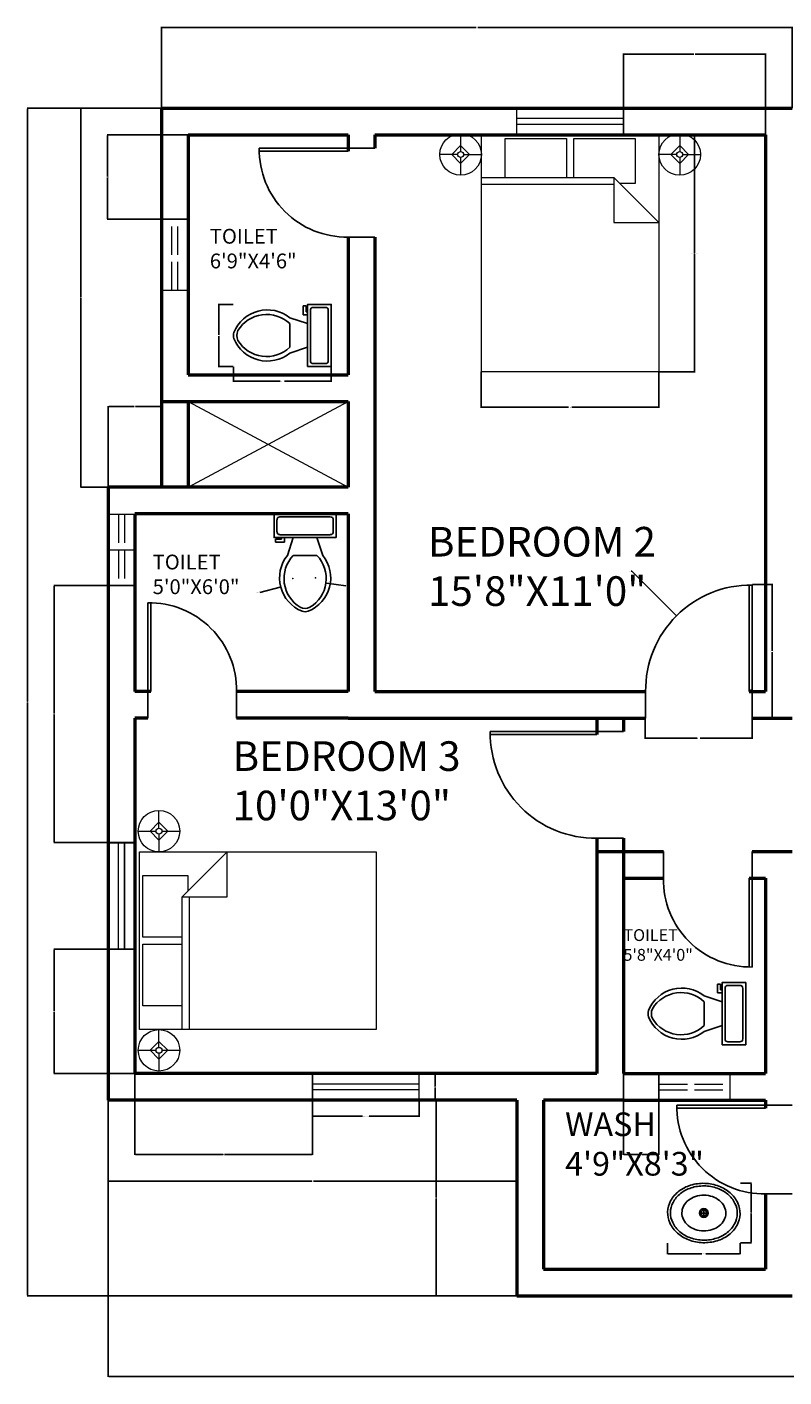
# Model space of a CAD drawing. Units: inches. Extents: x 178 to 719, y 262 to 748.
# Tile 1 of 3: x 178 to 434, y 292 to 748. Entities that reach past the tile are written whole.
import ezdxf

# ---------------------------------------------------------------- set-up
doc = ezdxf.new("R2010")
doc.units = ezdxf.units.IN
doc.linetypes.add('ACAD_ISO02W100', pattern=[15, 12, -3])
for name, color, linetype, lineweight in [('A-ANNO-DIMS', 2, 'Continuous', 18), ('A-AREA-IDEN', 7, 'Continuous', 25), ('A-DOOR', 3, 'Continuous', 25), ('A-FLOR-FIXT', 9, 'Continuous', 25), ('A-FLOR-OPEN', 8, 'Continuous', 18), ('A-FURN', 8, 'Continuous', 18), ('A-GLAZ', 4, 'Continuous', 18), ('A-GLAZ-OVHD', 4, 'ACAD_ISO02W100', 18), ('A-WALL', 7, 'Continuous', 50)]:
    doc.layers.add(name, color=color, linetype=linetype, lineweight=lineweight)
doc.styles.get("Standard").update_dxf_attribs({"font": 'arial.ttf'})
doc.dimstyles.get("Standard").update_dxf_attribs({"dimtxt": 0.18, "dimasz": 0.18, "dimexe": 0.18, "dimexo": 0.0625, "dimgap": 0.09, "dimtad": 0, "dimtih": 1, "dimtoh": 1, "dimdec": 4, "dimzin": 0, "dimdsep": 46, "dimtxsty": 'Standard', "dimcen": 0.09, "dimadec": 0, "dimazin": 0, "dimtfac": 1, "dimtdec": 4, "dimtofl": 0, "dimtmove": 0, "dimatfit": 3, "dimfxl": 1, "dimtolj": 1, "dimtzin": 0, "dimarcsym": 0})

# ---------------------------------------------------------------- blocks, each defined once
blk = doc.blocks.new('Toilet - top')
for p, q in [((9.5, -6), (9.5, -2)), ((-10, -8.5), (-8, -8.5)), ((-10, -9.5), (-10, -8.5)), ((-8, -8.5), (-8, -8)), ((-7, -8), (-7, -9.5)), ((-4, -8), (-6, -14)), ((4, -8), (6, -14)), ((-7, -9.5), (-10, -9.5)), ((4, -14), (-4, -14))]:
    blk.add_line(p, q)
blk.add_lwpolyline([(10.5, -8), (10.5, 0), (-10.5, 0), (-10.5, -8)], close=True)
for points in [[(-9.5, -2), (-9.5, -6)], [(8.5, -1), (-8.5, -1)], [(-8.5, -7), (8.5, -7)]]:
    blk.add_lwpolyline(points)
for centre, radius, start, end in [((-8.62, -1.88), 0.884, 81.8699, 188.1301), ((8.62, -1.88), 0.884, 351.8699, 98.1301), ((-8.62, -6.12), 0.884, 171.8699, 278.1301), ((8.62, -6.12), 0.884, 261.8699, 8.1301), ((3.52, -21.58), 12.17, 141.4691, 247.9714), ((4.2, -21.82), 11.33, 136.3677, 238.9468), ((-3.52, -21.58), 12.17, 292.0284, 38.5307), ((-4.2, -21.82), 11.33, 301.053, 43.6321), ((0, -27.88), 4, 245.7318, 294.2682), ((0, -29), 4, 254.8605, 285.1395)]:
    blk.add_arc(centre, radius, start, end)
blk = doc.blocks.new('Sink - Oval top')
for p, q in [((-1, 0), (1, 0)), ((0, 1), (0, -1))]:
    blk.add_line(p, q)
for points in [[(-12.23, 0.39, 0.117634), (-11.46, -3.36, 0.104469), (-8.88, -6.8, 0.090016), (-5.08, -9.07, 0.08192), (-0.32, -10.02, 0.08192), (4.49, -9.38, 0.090016), (8.42, -7.36, 0.104469), (11.22, -4.09, 0.117634), (12.23, -0.39, 0.117634), (11.46, 3.36, 0.104469), (8.88, 6.8, 0.090016), (5.08, 9.07, 0.08192), (0.32, 10.02, 0.08192), (-4.49, 9.38, 0.090016), (-8.42, 7.36, 0.104469), (-11.22, 4.09, 0.117634)], [(-11.29, 0.16, 0.118622), (-10.52, -3.25, 0.104678), (-8.07, -6.36, 0.089562), (-4.54, -8.37, 0.081185), (-0.13, -9.15, 0.081185), (4.3, -8.49, 0.089562), (7.89, -6.58, 0.104678), (10.42, -3.55, 0.118622), (11.29, -0.16, 0.118622), (10.52, 3.25, 0.104678), (8.07, 6.36, 0.089562), (4.54, 8.37, 0.081185), (0.13, 9.15, 0.081185), (-4.3, 8.49, 0.089562), (-7.89, 6.58, 0.104678), (-10.42, 3.55, 0.118622)], [(-7.42, 0.08, 0.118283), (-6.91, -2.17, 0.104607), (-5.29, -4.21, 0.089718), (-2.97, -5.53, 0.081436), (-0.07, -6.04, 0.081436), (2.84, -5.59, 0.089718), (5.2, -4.33, 0.104607), (6.86, -2.32, 0.118283), (7.42, -0.08, 0.118283), (6.91, 2.17, 0.104607), (5.29, 4.21, 0.089718), (2.97, 5.53, 0.081436), (0.07, 6.04, 0.081436), (-2.84, 5.59, 0.089718), (-5.2, 4.33, 0.104607), (-6.86, 2.32, 0.118283)]]:
    blk.add_lwpolyline(points, format="xyb", close=True)
for radius in [1.5, 1]:
    blk.add_circle((0, 0), radius)
blk = doc.blocks.new('Bed - Queen')
for p, q in [((0, -80.00003), (0, 0)), ((0, 0), (59.99999, 0)), ((59.99999, 0), (59.99999, -80.00003)), ((7.99999, -1.2), (28.79998, -1.2)), ((7.99999, -14.4), (7.99999, -1.2)), ((28.79998, -1.2), (28.79998, -14.4)), ((31.19999, -1.2), (51.99999, -1.2)), ((31.19999, -14.4), (31.19999, -1.2)), ((51.99999, -1.2), (51.99999, -16.4)), ((0, -14.4), (44.8, -14.4)), ((44.8, -16.8), (0, -16.8)), ((59.99999, -29.6), (44.8, -14.4)), ((44.8, -14.4), (44.8, -29.6)), ((51.99999, -16.4), (46.79936, -16.4)), ((44.8, -29.6), (59.99999, -29.6)), ((59.99999, -80.00003), (0, -80.00003))]:
    blk.add_line(p, q)
blk = doc.blocks.new('Lamp - Table')
for p, q in [((0, 7), (0, 1)), ((-1, 0), (-7, 0)), ((0, 3), (-3, 0)), ((-3, 0), (0, -3)), ((3, 0), (0, 3)), ((0, -3), (3, 0)), ((1, 0), (7, 0)), ((0, -1), (0, -7))]:
    blk.add_line(p, q)
for radius in [7, 1]:
    blk.add_circle((0, 0), radius)
blk = doc.blocks.new('DOOR-SWING-30IN')
for p, q in [((0, 0), (-30, 0)), ((0, 0), (9, 0)), ((0, -1), (-30, -1)), ((9, -30), (0, -30))]:
    blk.add_line(p, q)
blk.add_arc((-0.5, -0.5), 29.5, 179.029, 270.971)
blk = doc.blocks.new('DOOR-SWING-36IN')
for p, q in [((-1, 0), (-1, 36)), ((0, 0), (0, 36)), ((-36, 0), (-36, -9)), ((0, 0), (0, -9))]:
    blk.add_line(p, q)
blk.add_arc((-0.5, 0.5), 35.5, 89.1931, 180.8069)
blk = doc.blocks.new('WINDOW-36IN')
for p, q in [((0, 0), (0, 9)), ((36, 5.5), (0, 5.5)), ((36, 0), (36, 9)), ((36, 3.5), (0, 3.5))]:
    blk.add_line(p, q)
blk = doc.blocks.new('WINDOW-24IN-HIGH-GLAZING')
at = {"ltscale": 0.8}
for p, q in [((-2, 0), (-2, -24)), ((0, 0), (0, -24))]:
    blk.add_line(p, q, dxfattribs=at)
blk = doc.blocks.new('*D15')
at = {"layer": 'A-ANNO-DIMS', "color": 0, "lineweight": -2, "transparency": 16777216}
for p, q in [((391.76, 711.74), (403.88, 711.74)), ((403.7, 711.56), (403.7, 671.93)), ((403.7, 631.92), (403.7, 671.55)), ((391.76, 631.74), (403.88, 631.74))]:
    blk.add_line(p, q, dxfattribs=at)
at = {"layer": 'A-ANNO-DIMS', "color": 0, "transparency": 16777216}
for points in [[(403.67, 711.56), (403.73, 711.56), (403.7, 711.74)], [(403.67, 631.92), (403.73, 631.92), (403.7, 631.74)]]:
    blk.add_solid(points, dxfattribs=at)
at = {"layer": 'Defpoints', "color": 0, "transparency": 16777216}
for p in [(391.7, 711.74), (403.7, 711.74), (391.7, 631.74)]:
    blk.add_point(p, dxfattribs=at)
at = {"layer": 'A-ANNO-DIMS', "color": 0, "transparency": 16777216, "insert": (403.7, 671.74), "char_height": 0.18, "attachment_point": 5}
blk.add_mtext('\\A1;QUEEN BED 80 TYP.', dxfattribs=at)
blk = doc.blocks.new('*D16')
at = {"layer": 'A-ANNO-DIMS', "color": 0, "lineweight": -2, "transparency": 16777216}
for p, q in [((331.7, 631.67), (331.7, 619.56)), ((391.7, 631.67), (391.7, 619.56)), ((331.88, 619.74), (361.17, 619.74)), ((391.52, 619.74), (362.23, 619.74))]:
    blk.add_line(p, q, dxfattribs=at)
at = {"layer": 'A-ANNO-DIMS', "color": 0, "transparency": 16777216}
for points in [[(331.88, 619.77), (331.88, 619.71), (331.7, 619.74)], [(391.52, 619.77), (391.52, 619.71), (391.7, 619.74)]]:
    blk.add_solid(points, dxfattribs=at)
at = {"layer": 'Defpoints', "color": 0, "transparency": 16777216}
for p in [(331.7, 631.74), (391.7, 631.74), (391.7, 619.74)]:
    blk.add_point(p, dxfattribs=at)
at = {"layer": 'A-ANNO-DIMS', "color": 0, "transparency": 16777216, "insert": (361.7, 619.74), "char_height": 0.18, "attachment_point": 5}
blk.add_mtext('\\A1;60 TYP.', dxfattribs=at)
blk = doc.blocks.new('*D21')
at = {"layer": 'A-ANNO-DIMS', "color": 0, "lineweight": -2, "transparency": 16777216}
for p, q in [((423.26, 559.87), (430.15, 559.87)), ((429.97, 559.69), (429.97, 537.49)), ((429.97, 514.92), (429.97, 537.12)), ((423.26, 514.74), (430.15, 514.74))]:
    blk.add_line(p, q, dxfattribs=at)
at = {"layer": 'A-ANNO-DIMS', "color": 0, "transparency": 16777216}
for points in [[(429.94, 559.69), (430, 559.69), (429.97, 559.87)], [(429.94, 514.92), (430, 514.92), (429.97, 514.74)]]:
    blk.add_solid(points, dxfattribs=at)
at = {"layer": 'Defpoints', "color": 0, "transparency": 16777216}
for p in [(423.2, 559.87), (429.97, 559.87), (423.2, 514.74)]:
    blk.add_point(p, dxfattribs=at)
at = {"layer": 'A-ANNO-DIMS', "color": 0, "transparency": 16777216, "insert": (429.97, 537.3), "char_height": 0.18, "attachment_point": 5}
blk.add_mtext('\\A1;SWING DOOR 45 TYP.', dxfattribs=at)
blk = doc.blocks.new('*D22')
at = {"layer": 'A-ANNO-DIMS', "color": 0, "lineweight": -2, "transparency": 16777216}
for p, q in [((387.07, 514.67), (387.07, 507.79)), ((423.2, 514.67), (423.2, 507.79)), ((387.25, 507.97), (404.61, 507.97)), ((423.02, 507.97), (405.66, 507.97))]:
    blk.add_line(p, q, dxfattribs=at)
at = {"layer": 'A-ANNO-DIMS', "color": 0, "transparency": 16777216}
for points in [[(387.25, 508), (387.25, 507.94), (387.07, 507.97)], [(423.02, 508), (423.02, 507.94), (423.2, 507.97)]]:
    blk.add_solid(points, dxfattribs=at)
at = {"layer": 'Defpoints', "color": 0, "transparency": 16777216}
for p in [(387.07, 514.74), (423.2, 514.74), (423.2, 507.97)]:
    blk.add_point(p, dxfattribs=at)
at = {"layer": 'A-ANNO-DIMS', "color": 0, "transparency": 16777216, "insert": (405.13, 507.97), "char_height": 0.18, "attachment_point": 5}
blk.add_mtext('\\A1;36 TYP.', dxfattribs=at)
blk = doc.blocks.new('*D25')
at = {"layer": 'A-ANNO-DIMS', "color": 0, "lineweight": -2, "transparency": 16777216}
for p, q in [((274.7, 385.67), (274.7, 380.16)), ((310.7, 385.67), (310.7, 380.16)), ((274.88, 380.34), (291.58, 380.34)), ((310.52, 380.34), (293.82, 380.34))]:
    blk.add_line(p, q, dxfattribs=at)
at = {"layer": 'A-ANNO-DIMS', "color": 0, "transparency": 16777216}
for points in [[(274.88, 380.37), (274.88, 380.31), (274.7, 380.34)], [(310.52, 380.37), (310.52, 380.31), (310.7, 380.34)]]:
    blk.add_solid(points, dxfattribs=at)
at = {"layer": 'Defpoints', "color": 0, "transparency": 16777216}
for p in [(274.7, 385.74), (310.7, 385.74), (310.7, 380.34)]:
    blk.add_point(p, dxfattribs=at)
at = {"layer": 'A-ANNO-DIMS', "color": 0, "transparency": 16777216, "insert": (292.7, 380.34), "char_height": 0.18, "attachment_point": 5}
blk.add_mtext('\\A1;WINDOW 36 TYP.', dxfattribs=at)
blk = doc.blocks.new('*D26')
at = {"layer": 'A-ANNO-DIMS', "color": 0, "lineweight": -2, "transparency": 16777216}
for p, q in [((310.76, 394.74), (316.28, 394.74)), ((316.1, 394.56), (316.1, 390.42)), ((316.1, 385.92), (316.1, 390.06)), ((310.76, 385.74), (316.28, 385.74))]:
    blk.add_line(p, q, dxfattribs=at)
at = {"layer": 'A-ANNO-DIMS', "color": 0, "transparency": 16777216}
for points in [[(316.07, 394.56), (316.13, 394.56), (316.1, 394.74)], [(316.07, 385.92), (316.13, 385.92), (316.1, 385.74)]]:
    blk.add_solid(points, dxfattribs=at)
at = {"layer": 'Defpoints', "color": 0, "transparency": 16777216}
for p in [(310.7, 394.74), (316.1, 394.74), (310.7, 385.74)]:
    blk.add_point(p, dxfattribs=at)
at = {"layer": 'A-ANNO-DIMS', "color": 0, "transparency": 16777216, "insert": (316.1, 390.24), "char_height": 0.18, "attachment_point": 5}
blk.add_mtext('\\A1;9 TYP.', dxfattribs=at)
blk = doc.blocks.new('*D31')
at = {"layer": 'A-ANNO-DIMS', "color": 0, "lineweight": -2, "transparency": 16777216}
for p, q in [((247.95, 633.44), (247.95, 628.36)), ((281, 633.44), (281, 628.36)), ((248.13, 628.54), (263.7, 628.54)), ((280.82, 628.54), (265.25, 628.54))]:
    blk.add_line(p, q, dxfattribs=at)
at = {"layer": 'A-ANNO-DIMS', "color": 0, "transparency": 16777216}
for points in [[(248.13, 628.57), (248.13, 628.51), (247.95, 628.54)], [(280.82, 628.57), (280.82, 628.51), (281, 628.54)]]:
    blk.add_solid(points, dxfattribs=at)
at = {"layer": 'Defpoints', "color": 0, "transparency": 16777216}
for p in [(247.95, 633.5), (281, 633.5), (281, 628.54)]:
    blk.add_point(p, dxfattribs=at)
at = {"layer": 'A-ANNO-DIMS', "color": 0, "transparency": 16777216, "insert": (264.48, 628.54), "char_height": 0.18, "attachment_point": 5}
blk.add_mtext('\\A1;WC 33 TYP.', dxfattribs=at)
blk = doc.blocks.new('*D32')
at = {"layer": 'A-ANNO-DIMS', "color": 0, "lineweight": -2, "transparency": 16777216}
for p, q in [((247.89, 654.5), (242.82, 654.5)), ((243, 654.32), (243, 644.18)), ((243, 633.68), (243, 643.82)), ((247.89, 633.5), (242.82, 633.5))]:
    blk.add_line(p, q, dxfattribs=at)
at = {"layer": 'A-ANNO-DIMS', "color": 0, "transparency": 16777216}
for points in [[(242.97, 654.32), (243.03, 654.32), (243, 654.5)], [(242.97, 633.68), (243.03, 633.68), (243, 633.5)]]:
    blk.add_solid(points, dxfattribs=at)
at = {"layer": 'Defpoints', "color": 0, "transparency": 16777216}
for p in [(247.95, 654.5), (243, 633.5), (247.95, 633.5)]:
    blk.add_point(p, dxfattribs=at)
at = {"layer": 'A-ANNO-DIMS', "color": 0, "transparency": 16777216, "insert": (243, 644), "char_height": 0.18, "attachment_point": 5}
blk.add_mtext('\\A1;21 TYP.', dxfattribs=at)
blk = doc.blocks.new('*D35')
at = {"layer": 'A-ANNO-DIMS', "color": 0, "lineweight": -2, "transparency": 16777216}
for p, q in [((394.58, 337.55), (394.58, 333.75)), ((419.13, 337.55), (419.13, 333.75)), ((394.76, 333.93), (406.23, 333.93)), ((418.95, 333.93), (407.48, 333.93))]:
    blk.add_line(p, q, dxfattribs=at)
at = {"layer": 'A-ANNO-DIMS', "color": 0, "transparency": 16777216}
for points in [[(394.76, 333.96), (394.76, 333.9), (394.58, 333.93)], [(418.95, 333.96), (418.95, 333.9), (419.13, 333.93)]]:
    blk.add_solid(points, dxfattribs=at)
at = {"layer": 'Defpoints', "color": 0, "transparency": 16777216}
for p in [(394.58, 337.61), (419.13, 337.61), (419.13, 333.93)]:
    blk.add_point(p, dxfattribs=at)
at = {"layer": 'A-ANNO-DIMS', "color": 0, "transparency": 16777216, "insert": (406.86, 333.93), "char_height": 0.18, "attachment_point": 5}
blk.add_mtext('\\A1;BASIN 25', dxfattribs=at)
blk = doc.blocks.new('*D36')
at = {"layer": 'A-ANNO-DIMS', "color": 0, "lineweight": -2, "transparency": 16777216}
for p, q in [((419.19, 357.75), (422.99, 357.75)), ((422.81, 357.57), (422.81, 347.86)), ((422.81, 337.79), (422.81, 347.5)), ((419.19, 337.61), (422.99, 337.61))]:
    blk.add_line(p, q, dxfattribs=at)
at = {"layer": 'A-ANNO-DIMS', "color": 0, "transparency": 16777216}
for points in [[(422.78, 357.57), (422.84, 357.57), (422.81, 357.75)], [(422.78, 337.79), (422.84, 337.79), (422.81, 337.61)]]:
    blk.add_solid(points, dxfattribs=at)
at = {"layer": 'Defpoints', "color": 0, "transparency": 16777216}
for p in [(419.13, 357.75), (422.81, 357.75), (419.13, 337.61)]:
    blk.add_point(p, dxfattribs=at)
at = {"layer": 'A-ANNO-DIMS', "color": 0, "transparency": 16777216, "insert": (422.81, 347.68), "char_height": 0.18, "attachment_point": 5}
blk.add_mtext('\\A1;20', dxfattribs=at)
blk = doc.blocks.new('*D41')
at = {"layer": 'A-ANNO-DIMS', "color": 0, "lineweight": -2, "transparency": 16777216}
for p, q in [((205.7, 385.67), (205.7, 292.31)), ((691.7, 361.67), (691.7, 292.31)), ((205.88, 292.49), (448.41, 292.49)), ((691.52, 292.49), (448.99, 292.49))]:
    blk.add_line(p, q, dxfattribs=at)
at = {"layer": 'A-ANNO-DIMS', "color": 0, "transparency": 16777216}
for points in [[(205.88, 292.52), (205.88, 292.46), (205.7, 292.49)], [(691.52, 292.52), (691.52, 292.46), (691.7, 292.49)]]:
    blk.add_solid(points, dxfattribs=at)
at = {"layer": 'Defpoints', "color": 0, "transparency": 16777216}
for p in [(205.7, 385.74), (691.7, 361.74), (691.7, 292.49)]:
    blk.add_point(p, dxfattribs=at)
at = {"layer": 'A-ANNO-DIMS', "color": 0, "transparency": 16777216, "insert": (448.7, 292.49), "char_height": 0.18, "attachment_point": 5}
blk.add_mtext('\\A1;486', dxfattribs=at)
blk = doc.blocks.new('*D42')
at = {"layer": 'A-ANNO-DIMS', "color": 0, "lineweight": -2, "transparency": 16777216}
for p, q in [((223.64, 720.74), (178.27, 720.74)), ((178.45, 720.56), (178.45, 520.42)), ((178.45, 319.92), (178.45, 520.06)), ((343.64, 319.74), (178.27, 319.74))]:
    blk.add_line(p, q, dxfattribs=at)
at = {"layer": 'A-ANNO-DIMS', "color": 0, "transparency": 16777216}
for points in [[(178.42, 720.56), (178.48, 720.56), (178.45, 720.74)], [(178.42, 319.92), (178.48, 319.92), (178.45, 319.74)]]:
    blk.add_solid(points, dxfattribs=at)
at = {"layer": 'Defpoints', "color": 0, "transparency": 16777216}
for p in [(178.45, 720.74), (223.7, 720.74), (343.7, 319.74)]:
    blk.add_point(p, dxfattribs=at)
at = {"layer": 'A-ANNO-DIMS', "color": 0, "transparency": 16777216, "insert": (178.45, 520.24), "char_height": 0.18, "attachment_point": 5}
blk.add_mtext('\\A1;401', dxfattribs=at)
blk = doc.blocks.new('*D43')
at = {"layer": 'A-ANNO-DIMS', "color": 0, "lineweight": -2, "transparency": 16777216}
for p, q in [((205.7, 592.8), (205.7, 620.17)), ((205.88, 619.99), (214.49, 619.99)), ((223.52, 619.99), (214.91, 619.99)), ((223.7, 592.8), (223.7, 620.17))]:
    blk.add_line(p, q, dxfattribs=at)
at = {"layer": 'A-ANNO-DIMS', "color": 0, "transparency": 16777216}
for points in [[(205.88, 620.02), (205.88, 619.96), (205.7, 619.99)], [(223.52, 620.02), (223.52, 619.96), (223.7, 619.99)]]:
    blk.add_solid(points, dxfattribs=at)
at = {"layer": 'Defpoints', "color": 0, "transparency": 16777216}
for p in [(223.7, 619.99), (205.7, 592.74), (223.7, 592.74)]:
    blk.add_point(p, dxfattribs=at)
at = {"layer": 'A-ANNO-DIMS', "color": 0, "transparency": 16777216, "insert": (214.7, 619.99), "char_height": 0.18, "attachment_point": 5}
blk.add_mtext('\\A1;18', dxfattribs=at)
blk = doc.blocks.new('*D44')
at = {"layer": 'A-ANNO-DIMS', "color": 0, "lineweight": -2, "transparency": 16777216}
for p, q in [((223.7, 720.8), (223.7, 748.17)), ((223.88, 747.99), (329.91, 747.99)), ((436.52, 747.99), (330.49, 747.99)), ((436.7, 720.8), (436.7, 748.17))]:
    blk.add_line(p, q, dxfattribs=at)
at = {"layer": 'A-ANNO-DIMS', "color": 0, "transparency": 16777216}
for points in [[(223.88, 748.02), (223.88, 747.96), (223.7, 747.99)], [(436.52, 748.02), (436.52, 747.96), (436.7, 747.99)]]:
    blk.add_solid(points, dxfattribs=at)
at = {"layer": 'Defpoints', "color": 0, "transparency": 16777216}
for p in [(436.7, 747.99), (223.7, 720.74), (436.7, 720.74)]:
    blk.add_point(p, dxfattribs=at)
at = {"layer": 'A-ANNO-DIMS', "color": 0, "transparency": 16777216, "insert": (330.2, 747.99), "char_height": 0.18, "attachment_point": 5}
blk.add_mtext('\\A1;213', dxfattribs=at)
blk = doc.blocks.new('*D53')
at = {"layer": 'A-ANNO-DIMS', "color": 0, "lineweight": -2, "transparency": 16777216}
for p, q in [((205.7, 385.67), (205.7, 358.31)), ((343.7, 385.67), (343.7, 358.31)), ((205.88, 358.49), (274.42, 358.49)), ((343.52, 358.49), (274.98, 358.49))]:
    blk.add_line(p, q, dxfattribs=at)
at = {"layer": 'A-ANNO-DIMS', "color": 0, "transparency": 16777216}
for points in [[(205.88, 358.52), (205.88, 358.46), (205.7, 358.49)], [(343.52, 358.52), (343.52, 358.46), (343.7, 358.49)]]:
    blk.add_solid(points, dxfattribs=at)
at = {"layer": 'Defpoints', "color": 0, "transparency": 16777216}
for p in [(205.7, 385.74), (343.7, 385.74), (205.7, 358.49)]:
    blk.add_point(p, dxfattribs=at)
at = {"layer": 'A-ANNO-DIMS', "color": 0, "transparency": 16777216, "insert": (274.7, 358.49), "char_height": 0.18, "attachment_point": 5}
blk.add_mtext('\\A1;138', dxfattribs=at)
blk = doc.blocks.new('*D55')
at = {"layer": 'A-ANNO-DIMS', "color": 0, "lineweight": -2, "transparency": 16777216}
for p, q in [((343.64, 385.74), (316.27, 385.74)), ((316.45, 385.56), (316.45, 352.92)), ((316.45, 319.92), (316.45, 352.56)), ((343.64, 319.74), (316.27, 319.74))]:
    blk.add_line(p, q, dxfattribs=at)
at = {"layer": 'A-ANNO-DIMS', "color": 0, "transparency": 16777216}
for points in [[(316.42, 385.56), (316.48, 385.56), (316.45, 385.74)], [(316.42, 319.92), (316.48, 319.92), (316.45, 319.74)]]:
    blk.add_solid(points, dxfattribs=at)
at = {"layer": 'Defpoints', "color": 0, "transparency": 16777216}
for p in [(316.45, 385.74), (343.7, 385.74), (343.7, 319.74)]:
    blk.add_point(p, dxfattribs=at)
at = {"layer": 'A-ANNO-DIMS', "color": 0, "transparency": 16777216, "insert": (316.45, 352.74), "char_height": 0.18, "attachment_point": 5}
blk.add_mtext('\\A1;66', dxfattribs=at)
blk = doc.blocks.new('*D56')
at = {"layer": 'A-ANNO-DIMS', "color": 0, "lineweight": -2, "transparency": 16777216}
for p, q in [((223.64, 720.74), (196.27, 720.74)), ((196.45, 720.56), (196.45, 656.92)), ((196.45, 592.92), (196.45, 656.56)), ((223.64, 592.74), (196.27, 592.74))]:
    blk.add_line(p, q, dxfattribs=at)
at = {"layer": 'A-ANNO-DIMS', "color": 0, "transparency": 16777216}
for points in [[(196.42, 720.56), (196.48, 720.56), (196.45, 720.74)], [(196.42, 592.92), (196.48, 592.92), (196.45, 592.74)]]:
    blk.add_solid(points, dxfattribs=at)
at = {"layer": 'Defpoints', "color": 0, "transparency": 16777216}
for p in [(196.45, 720.74), (223.7, 720.74), (223.7, 592.74)]:
    blk.add_point(p, dxfattribs=at)
at = {"layer": 'A-ANNO-DIMS', "color": 0, "transparency": 16777216, "insert": (196.45, 656.74), "char_height": 0.18, "attachment_point": 5}
blk.add_mtext('\\A1;128', dxfattribs=at)
blk = doc.blocks.new('*D57')
at = {"layer": 'A-ANNO-DIMS', "color": 0, "lineweight": -2, "transparency": 16777216}
for p, q in [((379.7, 711.8), (379.7, 739.17)), ((379.88, 738.99), (403.48, 738.99)), ((427.52, 738.99), (403.92, 738.99)), ((427.7, 711.8), (427.7, 739.17))]:
    blk.add_line(p, q, dxfattribs=at)
at = {"layer": 'A-ANNO-DIMS', "color": 0, "transparency": 16777216}
for points in [[(379.88, 739.02), (379.88, 738.96), (379.7, 738.99)], [(427.52, 739.02), (427.52, 738.96), (427.7, 738.99)]]:
    blk.add_solid(points, dxfattribs=at)
at = {"layer": 'Defpoints', "color": 0, "transparency": 16777216}
for p in [(427.7, 738.99), (379.7, 711.74), (427.7, 711.74)]:
    blk.add_point(p, dxfattribs=at)
at = {"layer": 'A-ANNO-DIMS', "color": 0, "transparency": 16777216, "insert": (403.7, 738.99), "char_height": 0.18, "attachment_point": 5}
blk.add_mtext('\\A1;48', dxfattribs=at)
blk = doc.blocks.new('*D59')
at = {"layer": 'A-ANNO-DIMS', "color": 0, "lineweight": -2, "transparency": 16777216}
for p, q in [((214.7, 394.67), (214.7, 367.31)), ((274.7, 394.67), (274.7, 367.31)), ((214.88, 367.49), (244.48, 367.49)), ((274.52, 367.49), (244.92, 367.49))]:
    blk.add_line(p, q, dxfattribs=at)
at = {"layer": 'A-ANNO-DIMS', "color": 0, "transparency": 16777216}
for points in [[(214.88, 367.52), (214.88, 367.46), (214.7, 367.49)], [(274.52, 367.52), (274.52, 367.46), (274.7, 367.49)]]:
    blk.add_solid(points, dxfattribs=at)
at = {"layer": 'Defpoints', "color": 0, "transparency": 16777216}
for p in [(214.7, 394.74), (274.7, 394.74), (214.7, 367.49)]:
    blk.add_point(p, dxfattribs=at)
at = {"layer": 'A-ANNO-DIMS', "color": 0, "transparency": 16777216, "insert": (244.7, 367.49), "char_height": 0.18, "attachment_point": 5}
blk.add_mtext('\\A1;60', dxfattribs=at)
blk = doc.blocks.new('*D64')
at = {"layer": 'A-ANNO-DIMS', "color": 0, "lineweight": -2, "transparency": 16777216}
for p, q in [((214.64, 436.74), (187.27, 436.74)), ((187.45, 436.56), (187.45, 415.92)), ((187.45, 394.92), (187.45, 415.56)), ((214.64, 394.74), (187.27, 394.74))]:
    blk.add_line(p, q, dxfattribs=at)
at = {"layer": 'A-ANNO-DIMS', "color": 0, "transparency": 16777216}
for points in [[(187.42, 436.56), (187.48, 436.56), (187.45, 436.74)], [(187.42, 394.92), (187.48, 394.92), (187.45, 394.74)]]:
    blk.add_solid(points, dxfattribs=at)
at = {"layer": 'Defpoints', "color": 0, "transparency": 16777216}
for p in [(187.45, 436.74), (214.7, 436.74), (214.7, 394.74)]:
    blk.add_point(p, dxfattribs=at)
at = {"layer": 'A-ANNO-DIMS', "color": 0, "transparency": 16777216, "insert": (187.45, 415.74), "char_height": 0.18, "attachment_point": 5}
blk.add_mtext('\\A1;42', dxfattribs=at)
blk = doc.blocks.new('*D65')
at = {"layer": 'A-ANNO-DIMS', "color": 0, "lineweight": -2, "transparency": 16777216}
for p, q in [((214.64, 559.54), (187.27, 559.54)), ((187.45, 559.36), (187.45, 516.32)), ((187.45, 472.92), (187.45, 515.96)), ((214.64, 472.74), (187.27, 472.74))]:
    blk.add_line(p, q, dxfattribs=at)
at = {"layer": 'A-ANNO-DIMS', "color": 0, "transparency": 16777216}
for points in [[(187.42, 559.36), (187.48, 559.36), (187.45, 559.54)], [(187.42, 472.92), (187.48, 472.92), (187.45, 472.74)]]:
    blk.add_solid(points, dxfattribs=at)
at = {"layer": 'Defpoints', "color": 0, "transparency": 16777216}
for p in [(187.45, 559.54), (214.7, 559.54), (214.7, 472.74)]:
    blk.add_point(p, dxfattribs=at)
at = {"layer": 'A-ANNO-DIMS', "color": 0, "transparency": 16777216, "insert": (187.45, 516.14), "char_height": 0.18, "attachment_point": 5}
blk.add_mtext('\\A1;86.8', dxfattribs=at)
blk = doc.blocks.new('*D66')
at = {"layer": 'A-ANNO-DIMS', "color": 0, "lineweight": -2, "transparency": 16777216}
for p, q in [((232.64, 711.74), (205.27, 711.74)), ((205.45, 711.56), (205.45, 697.67)), ((205.45, 683.42), (205.45, 697.31)), ((232.64, 683.24), (205.27, 683.24))]:
    blk.add_line(p, q, dxfattribs=at)
at = {"layer": 'A-ANNO-DIMS', "color": 0, "transparency": 16777216}
for points in [[(205.42, 711.56), (205.48, 711.56), (205.45, 711.74)], [(205.42, 683.42), (205.48, 683.42), (205.45, 683.24)]]:
    blk.add_solid(points, dxfattribs=at)
at = {"layer": 'Defpoints', "color": 0, "transparency": 16777216}
for p in [(205.45, 711.74), (232.7, 711.74), (232.7, 683.24)]:
    blk.add_point(p, dxfattribs=at)
at = {"layer": 'A-ANNO-DIMS', "color": 0, "transparency": 16777216, "insert": (205.45, 697.49), "char_height": 0.18, "attachment_point": 5}
blk.add_mtext('\\A1;28.5', dxfattribs=at)
blk = doc.blocks.new('*D69')
at = {"layer": 'A-ANNO-DIMS', "color": 0, "lineweight": -2, "transparency": 16777216}
for p, q in [((379.7, 394.67), (379.7, 367.31)), ((391.7, 394.67), (391.7, 367.31)), ((379.88, 367.49), (385.49, 367.49)), ((391.52, 367.49), (385.91, 367.49))]:
    blk.add_line(p, q, dxfattribs=at)
at = {"layer": 'A-ANNO-DIMS', "color": 0, "transparency": 16777216}
for points in [[(379.88, 367.52), (379.88, 367.46), (379.7, 367.49)], [(391.52, 367.52), (391.52, 367.46), (391.7, 367.49)]]:
    blk.add_solid(points, dxfattribs=at)
at = {"layer": 'Defpoints', "color": 0, "transparency": 16777216}
for p in [(379.7, 394.74), (391.7, 394.74), (379.7, 367.49)]:
    blk.add_point(p, dxfattribs=at)
at = {"layer": 'A-ANNO-DIMS', "color": 0, "transparency": 16777216, "insert": (385.7, 367.49), "char_height": 0.18, "attachment_point": 5}
blk.add_mtext('\\A1;12', dxfattribs=at)
blk = doc.blocks.new('*D70')
at = {"layer": 'A-ANNO-DIMS', "color": 0, "lineweight": -2, "transparency": 16777216}
for p, q in [((382.35, 564.4), (382.53, 564.4)), ((382.53, 564.4), (397.47, 549.47)), ((422.7, 524.15), (422.7, 524.33)), ((422.61, 524.24), (422.79, 524.24))]:
    blk.add_line(p, q, dxfattribs=at)
at = {"layer": 'A-ANNO-DIMS', "color": 0, "transparency": 16777216}
blk.add_solid([(397.49, 549.49), (397.45, 549.45), (397.6, 549.34)], dxfattribs=at)
at = {"layer": 'Defpoints', "color": 0, "transparency": 16777216}
for p in [(397.6, 549.34), (422.7, 524.24)]:
    blk.add_point(p, dxfattribs=at)
at = {"layer": 'A-ANNO-DIMS', "color": 0, "transparency": 16777216, "insert": (381.75, 564.4), "char_height": 0.18, "attachment_point": 5}
blk.add_mtext('\\A1;3X R35.5', dxfattribs=at)
blk = doc.blocks.new('*D76')
at = {"layer": 'A-ANNO-DIMS', "color": 0, "lineweight": -2, "transparency": 16777216}
for p, q in [((275.61, 562.16), (275.79, 562.16)), ((275.7, 562.07), (275.7, 562.25)), ((256.87, 557.21), (263.76, 559.02))]:
    blk.add_line(p, q, dxfattribs=at)
at = {"layer": 'A-ANNO-DIMS', "color": 0, "transparency": 16777216}
blk.add_solid([(263.75, 559.05), (263.77, 558.99), (263.94, 559.06)], dxfattribs=at)
at = {"layer": 'Defpoints', "color": 0, "transparency": 16777216}
for p in [(275.7, 562.16), (263.94, 559.06)]:
    blk.add_point(p, dxfattribs=at)
at = {"layer": 'A-ANNO-DIMS', "color": 0, "transparency": 16777216, "insert": (256.2, 557.21), "char_height": 0.18, "attachment_point": 5}
blk.add_mtext('\\A1;6X R12.17', dxfattribs=at)
blk = doc.blocks.new('*D77')
at = {"layer": 'A-ANNO-DIMS', "color": 0, "lineweight": -2, "transparency": 16777216}
for p, q in [((267.9, 561.92), (268.08, 561.92)), ((267.99, 561.83), (267.99, 562.01)), ((285.95, 559.5), (279.39, 560.39))]:
    blk.add_line(p, q, dxfattribs=at)
at = {"layer": 'A-ANNO-DIMS', "color": 0, "transparency": 16777216}
blk.add_solid([(279.4, 560.42), (279.39, 560.36), (279.21, 560.41)], dxfattribs=at)
at = {"layer": 'Defpoints', "color": 0, "transparency": 16777216}
for p in [(267.99, 561.92), (279.21, 560.41)]:
    blk.add_point(p, dxfattribs=at)
at = {"layer": 'A-ANNO-DIMS', "color": 0, "transparency": 16777216, "insert": (286.62, 559.5), "char_height": 0.18, "attachment_point": 5}
blk.add_mtext('\\A1;6X R11.33', dxfattribs=at)

msp = doc.modelspace()

# ---------------------------------------------------------------- linework, layer by layer
at = {"layer": 'A-FLOR-OPEN'}
for p, q in [((232.7008, 592.737), (286.7008, 621.737)), ((232.7008, 621.737), (286.7008, 592.737))]:
    msp.add_line(p, q, dxfattribs=at)
at = {"layer": 'A-GLAZ'}
for p, q in [((232.7008, 683.237), (223.7008, 683.237)), ((232.7008, 659.237), (223.7008, 659.237)), ((214.7008, 583.5376), (205.7008, 583.5376)), ((214.7008, 571.5376), (205.7008, 571.5376)), ((214.7008, 559.5376), (205.7008, 559.5376)), ((211.2008, 472.737), (211.2008, 436.737)), ((211.2008, 472.737), (211.2008, 436.737)), ((391.7008, 385.737), (391.7008, 394.737)), ((415.7008, 385.737), (415.7008, 394.737))]:
    msp.add_line(p, q, dxfattribs=at)
at = {"layer": 'A-WALL'}
for p, q in [((223.7008, 720.737), (223.7008, 592.737)), ((223.7008, 720.737), (295.7008, 720.737)), ((295.7008, 720.737), (436.7008, 720.737)), ((232.7008, 711.737), (232.7008, 630.737)), ((232.7008, 711.737), (286.7008, 711.737)), ((286.7008, 711.737), (286.7008, 706.237)), ((295.7008, 711.737), (295.7008, 707.237)), ((295.7008, 711.737), (427.7008, 711.737)), ((427.7008, 711.737), (427.7008, 523.737)), ((286.7008, 677.237), (286.7008, 630.737)), ((295.7008, 677.237), (295.7008, 523.737)), ((232.7008, 630.737), (286.7008, 630.737)), ((223.7008, 621.737), (286.7008, 621.737)), ((232.7008, 621.737), (232.7008, 592.737)), ((286.7008, 621.737), (286.7008, 592.737)), ((205.7008, 592.737), (205.7008, 514.737)), ((286.7008, 592.737), (205.7008, 592.737)), ((214.7008, 583.737), (214.7008, 523.737)), ((286.7008, 583.737), (214.7008, 583.737)), ((286.7008, 583.737), (286.7008, 523.737)), ((220.0222, 523.737), (214.7008, 523.737)), ((286.7008, 523.737), (249.0222, 523.737)), ((295.7008, 523.737), (387.2008, 523.737)), ((422.2008, 523.737), (427.7008, 523.737)), ((205.7008, 514.737), (205.7008, 385.737)), ((214.7008, 514.737), (214.7008, 394.737)), ((219.0222, 514.737), (214.7008, 514.737)), ((286.7008, 514.737), (249.0222, 514.737)), ((286.7008, 514.737), (370.7008, 514.737)), ((370.7008, 514.737), (370.7008, 509.237)), ((370.7008, 514.737), (387.2008, 514.737)), ((379.7008, 514.737), (379.7008, 510.237)), ((423.2008, 514.737), (436.7008, 514.737)), ((370.7008, 474.237), (370.7008, 394.737)), ((379.7008, 474.237), (379.7008, 394.737)), ((370.7008, 469.737), (393.2008, 469.737)), ((423.2008, 469.737), (436.7008, 469.737)), ((379.7008, 460.737), (393.2008, 460.737)), ((422.2008, 460.737), (427.7008, 460.737)), ((427.7008, 460.737), (427.7008, 394.737)), ((370.7008, 394.737), (214.7008, 394.737)), ((379.7008, 394.737), (427.7008, 394.737)), ((343.7008, 385.737), (205.7008, 385.737)), ((343.7008, 385.737), (343.7008, 319.737)), ((379.7008, 385.737), (352.7008, 385.737)), ((352.7008, 385.737), (352.7008, 328.737)), ((379.7008, 385.737), (427.7008, 385.737)), ((427.7008, 385.737), (427.7008, 383.1411)), ((427.7008, 354.1411), (427.7008, 328.737)), ((352.7008, 328.737), (427.7008, 328.737)), ((343.7008, 319.737), (436.7008, 319.737))]:
    msp.add_line(p, q, dxfattribs=at)

# ---------------------------------------------------------------- block references
at = {"layer": 'A-DOOR'}
for name, p in [('DOOR-SWING-30IN', (286.7008, 707.237)), ('DOOR-SWING-36IN', (423.2008, 523.737)), ('DOOR-SWING-30IN', (427.7008, 384.1411))]:
    msp.add_blockref(name, p, dxfattribs=at)
at = {"layer": 'A-DOOR', "extrusion": (0, 0, -1), "zscale": -1}
for p, rotation in [((-219.0222, 523.737), 269.9999999999996), ((-423.2008, 460.737), 90.00000000000115)]:
    msp.add_blockref('DOOR-SWING-30IN', p, dxfattribs=dict(at, rotation=rotation))
at = {"layer": 'A-DOOR', "rotation": 90.00000000000003}
msp.add_blockref('DOOR-SWING-36IN', (370.7008, 510.237), dxfattribs=at)
at = {"layer": 'A-FLOR-FIXT', "rotation": 270}
for p in [(281, 644), (421, 415)]:
    msp.add_blockref('Toilet - top', p, dxfattribs=at)
at = {"layer": 'A-FLOR-FIXT'}
for name, p in [('Toilet - top', (272.1853, 583.737)), ('Sink - Oval top', (406.8569, 347.6786))]:
    msp.add_blockref(name, p, dxfattribs=at)
at = {"layer": 'A-FURN'}
for name, p in [('Lamp - Table', (324.7036, 705.1157)), ('Bed - Queen', (331.7008, 711.737)), ('Lamp - Table', (398.7008, 705.1157))]:
    msp.add_blockref(name, p, dxfattribs=at)
at = {"layer": 'A-FURN', "rotation": 90}
for name, p in [('Lamp - Table', (222.8221, 476.6178)), ('Bed - Queen', (216.2008, 409.6178)), ('Lamp - Table', (222.8221, 402.6206))]:
    msp.add_blockref(name, p, dxfattribs=at)
at = {"layer": 'A-GLAZ'}
for p in [(343.7008, 711.737), (274.7008, 385.737)]:
    msp.add_blockref('WINDOW-36IN', p, dxfattribs=at)
at = {"layer": 'A-GLAZ', "rotation": 270.0000000000002}
msp.add_blockref('WINDOW-36IN', (205.7008, 472.737), dxfattribs=at)
at = {"layer": 'A-GLAZ-OVHD'}
for p, rotation in [((227.2008, 659.237), 180), ((391.7008, 391.237), 90)]:
    msp.add_blockref('WINDOW-24IN-HIGH-GLAZING', p, dxfattribs=dict(at, rotation=rotation))
msp.add_blockref('WINDOW-24IN-HIGH-GLAZING', (211.2008, 583.5376), dxfattribs=at)

# ---------------------------------------------------------------- texts
at = {"layer": 'A-AREA-IDEN', "attachment_point": 1}
for s, width, insert, char_height in [('TOILET\\P6\'9"X4\'6"', 30, (240, 680), 5), ('BEDROOM 2\\P15\'8"X11\'0"', 98.987328, (313.6744, 579.3564), 10), ('TOILET\\P5\'0"X6\'0"', 30, (220.7008, 570), 5), ('BEDROOM 3\\P10\'0"X13\'0"', 98.987328, (247.6828, 506.9602), 10), ('TOILET\\P5\'8"X4\'0"', 30, (379.7008, 443.5277), 4), ('WASH\\P4\'9"X8\'3"', 98.987328, (360, 381.6444), 8)]:
    msp.add_mtext_dynamic_manual_height_columns(s, width=width, gutter_width=12.5, heights=[0], dxfattribs=dict(at, insert=insert, char_height=char_height))

# ---------------------------------------------------------------- dimensions: what is measured, and where the dimension line sits
at = {"layer": 'A-ANNO-DIMS'}
for base, p1, p2, picture, middle in [((436.7008, 747.987), (223.7008, 720.737), (436.7008, 720.737), '*D44', (330.2008, 747.987)), ((427.7008, 738.987), (379.7008, 711.737), (427.7008, 711.737), '*D57', (403.7008, 738.987)), ((691.7008, 292.487), (205.7008, 385.737), (691.7008, 361.737), '*D41', (448.7008, 292.487))]:
    dim = msp.add_linear_dim(base=base, p1=p1, p2=p2, dimstyle='Standard', override={"dimdec": 0, "dimlfac": 1, "dimrnd": 0, "dimzin": 0, "dimdsep": 46, "dimlunit": 2}, dxfattribs=at)
    dim.commit()
    dim.dimension.update_dxf_attribs({"geometry": picture, "text_midpoint": middle})
for base, p1, p2, angle, override, picture, middle in [((178.4508, 720.737), (343.7008, 319.737), (223.7008, 720.737), 90, {"dimdec": 0, "dimlfac": 1, "dimrnd": 0, "dimzin": 0, "dimdsep": 46, "dimlunit": 2}, '*D42', (178.4508, 520.237)), ((196.4508, 720.737), (223.7008, 592.737), (223.7008, 720.737), 90, {"dimdec": 0, "dimlfac": 1, "dimrnd": 0, "dimzin": 0, "dimdsep": 46, "dimlunit": 2}, '*D56', (196.4508, 656.737)), ((205.4508, 711.737), (232.7008, 683.237), (232.7008, 711.737), 90, {"dimdec": 1, "dimlfac": 1, "dimrnd": 0, "dimzin": 0, "dimdsep": 46, "dimlunit": 2}, '*D66', (205.4508, 697.487)), ((223.7008, 619.987), (205.7008, 592.737), (223.7008, 592.737), 0, {"dimdec": 0, "dimlfac": 1, "dimrnd": 0, "dimzin": 0, "dimdsep": 46, "dimlunit": 2}, '*D43', (214.7008, 619.987)), ((187.4508, 559.5376), (214.7008, 472.737), (214.7008, 559.5376), 90, {"dimdec": 1, "dimlfac": 1, "dimrnd": 0, "dimzin": 0, "dimdsep": 46, "dimlunit": 2}, '*D65', (187.4508, 516.1373)), ((187.4508, 436.737), (214.7008, 394.737), (214.7008, 436.737), 90, {"dimdec": 0, "dimlfac": 1, "dimrnd": 0, "dimzin": 0, "dimdsep": 46, "dimlunit": 2}, '*D64', (187.4508, 415.737)), ((214.7008, 367.487), (274.7008, 394.737), (214.7008, 394.737), 180, {"dimdec": 0, "dimlfac": 1, "dimrnd": 0, "dimzin": 0, "dimdsep": 46, "dimlunit": 2}, '*D59', (244.7008, 367.487)), ((379.7008, 367.487), (391.7008, 394.737), (379.7008, 394.737), 180, {"dimdec": 0, "dimlfac": 1, "dimrnd": 0, "dimzin": 0, "dimdsep": 46, "dimlunit": 2}, '*D69', (385.7008, 367.487)), ((205.7008, 358.487), (343.7008, 385.737), (205.7008, 385.737), 180, {"dimdec": 0, "dimlfac": 1, "dimrnd": 0, "dimzin": 0, "dimdsep": 46, "dimlunit": 2}, '*D53', (274.7008, 358.487)), ((316.4508, 385.737), (343.7008, 319.737), (343.7008, 385.737), 90, {"dimdec": 0, "dimlfac": 1, "dimrnd": 0, "dimzin": 0, "dimdsep": 46, "dimlunit": 2}, '*D55', (316.4508, 352.737)), ((422.8149, 357.7469), (419.1323, 337.6103), (419.1323, 357.7469), 90, {"dimdec": 0, "dimlfac": 1, "dimrnd": 0, "dimzin": 0, "dimdsep": 46, "dimlunit": 2}, '*D36', (422.8149, 347.6786))]:
    dim = msp.add_linear_dim(base=base, p1=p1, p2=p2, angle=angle, dimstyle='Standard', override=override, dxfattribs=at)
    dim.commit()
    dim.dimension.update_dxf_attribs({"geometry": picture, "text_midpoint": middle})
for base, p1, p2, angle, text, picture, middle in [((403.7008, 711.737), (391.7008, 631.737), (391.7008, 711.737), 90, 'QUEEN BED <> TYP.', '*D15', (403.7008, 671.737)), ((242.9968, 633.5), (247.9538, 654.5), (247.9538, 633.5), 270, '<> TYP.', '*D32', (242.9968, 644)), ((429.9711, 559.872), (423.2008, 514.737), (423.2008, 559.872), 90, 'SWING DOOR <> TYP.', '*D21', (429.9711, 537.3045)), ((316.1008, 394.737), (310.7008, 385.737), (310.7008, 394.737), 90, '<> TYP.', '*D26', (316.1008, 390.237))]:
    dim = msp.add_linear_dim(base=base, p1=p1, p2=p2, angle=angle, text=text, dimstyle='Standard', override={"dimdec": 0, "dimlfac": 1, "dimrnd": 0, "dimzin": 0, "dimdsep": 46, "dimlunit": 2}, dxfattribs=at)
    dim.commit()
    dim.dimension.update_dxf_attribs({"geometry": picture, "text_midpoint": middle})
for base, p1, p2, text, picture, middle in [((281, 628.5431), (247.9538, 633.5), (281, 633.5), 'WC <> TYP.', '*D31', (264.4769, 628.5431)), ((391.7008, 619.737), (331.7008, 631.737), (391.7008, 631.737), '<> TYP.', '*D16', (361.7008, 619.737)), ((423.2008, 507.9667), (387.0658, 514.737), (423.2008, 514.737), '<> TYP.', '*D22', (405.1333, 507.9667)), ((310.7008, 380.337), (274.7008, 385.737), (310.7008, 385.737), 'WINDOW <> TYP.', '*D25', (292.7008, 380.337)), ((419.1323, 333.9277), (394.5814, 337.6103), (419.1323, 337.6103), 'BASIN <>', '*D35', (406.8569, 333.9277))]:
    dim = msp.add_linear_dim(base=base, p1=p1, p2=p2, text=text, dimstyle='Standard', override={"dimdec": 0, "dimlfac": 1, "dimrnd": 0, "dimzin": 0, "dimdsep": 46, "dimlunit": 2}, dxfattribs=at)
    dim.commit()
    dim.dimension.update_dxf_attribs({"geometry": picture, "text_midpoint": middle})
for center, mpoint, text, override, picture, middle in [((275.7049, 562.1565), (263.9354, 559.0641), '6X <>', {"dimdec": 2, "dimlfac": 1, "dimrnd": 0, "dimzin": 0, "dimdsep": 46, "dimlunit": 2}, '*D76', (256.8736, 557.2087)), ((267.9854, 561.9196), (279.2136, 560.4101), '6X <>', {"dimdec": 2, "dimlfac": 1, "dimrnd": 0, "dimzin": 0, "dimdsep": 46, "dimlunit": 2}, '*D77', (285.9505, 559.5043)), ((422.7008, 524.237), (397.5961, 549.3419), '3X <>', {"dimdec": 1, "dimlfac": 1, "dimrnd": 0, "dimzin": 0, "dimdsep": 46, "dimlunit": 2}, '*D70', (381.7494, 564.4048))]:
    dim = msp.add_radius_dim(center=center, mpoint=mpoint, text=text, dimstyle='Standard', override=override, dxfattribs=at)
    dim.commit()
    dim.dimension.update_dxf_attribs({"geometry": picture, "text_midpoint": middle, "dimtype": 164})

doc.saveas('drawing.dxf')
